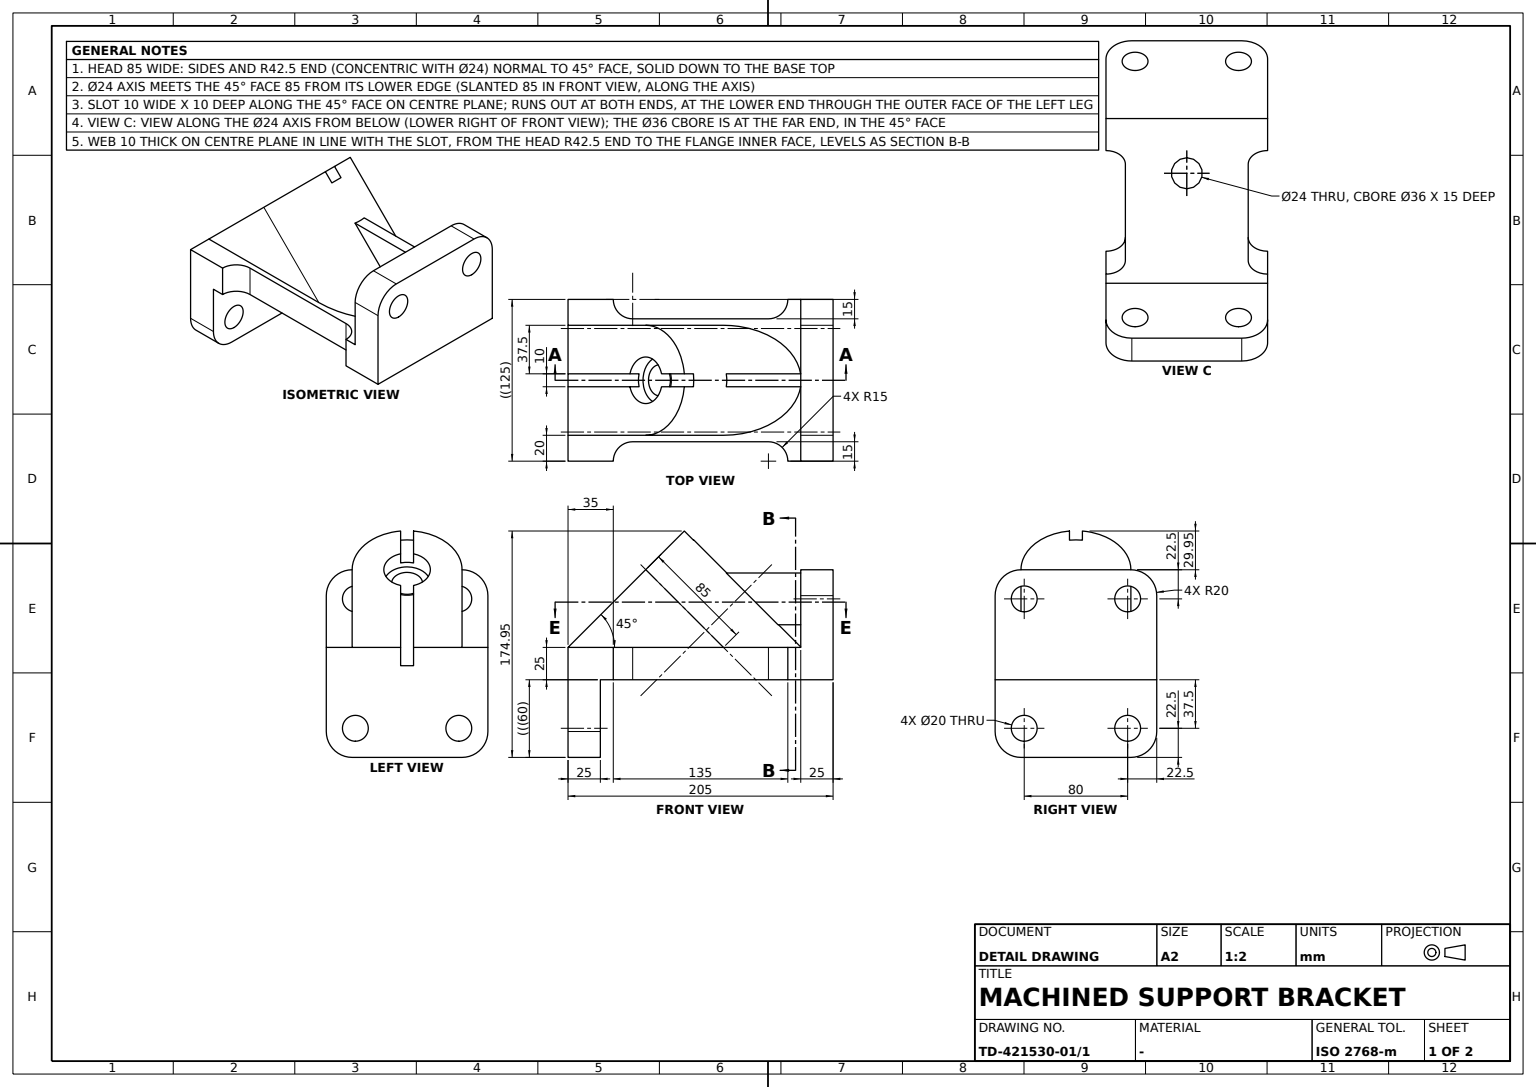
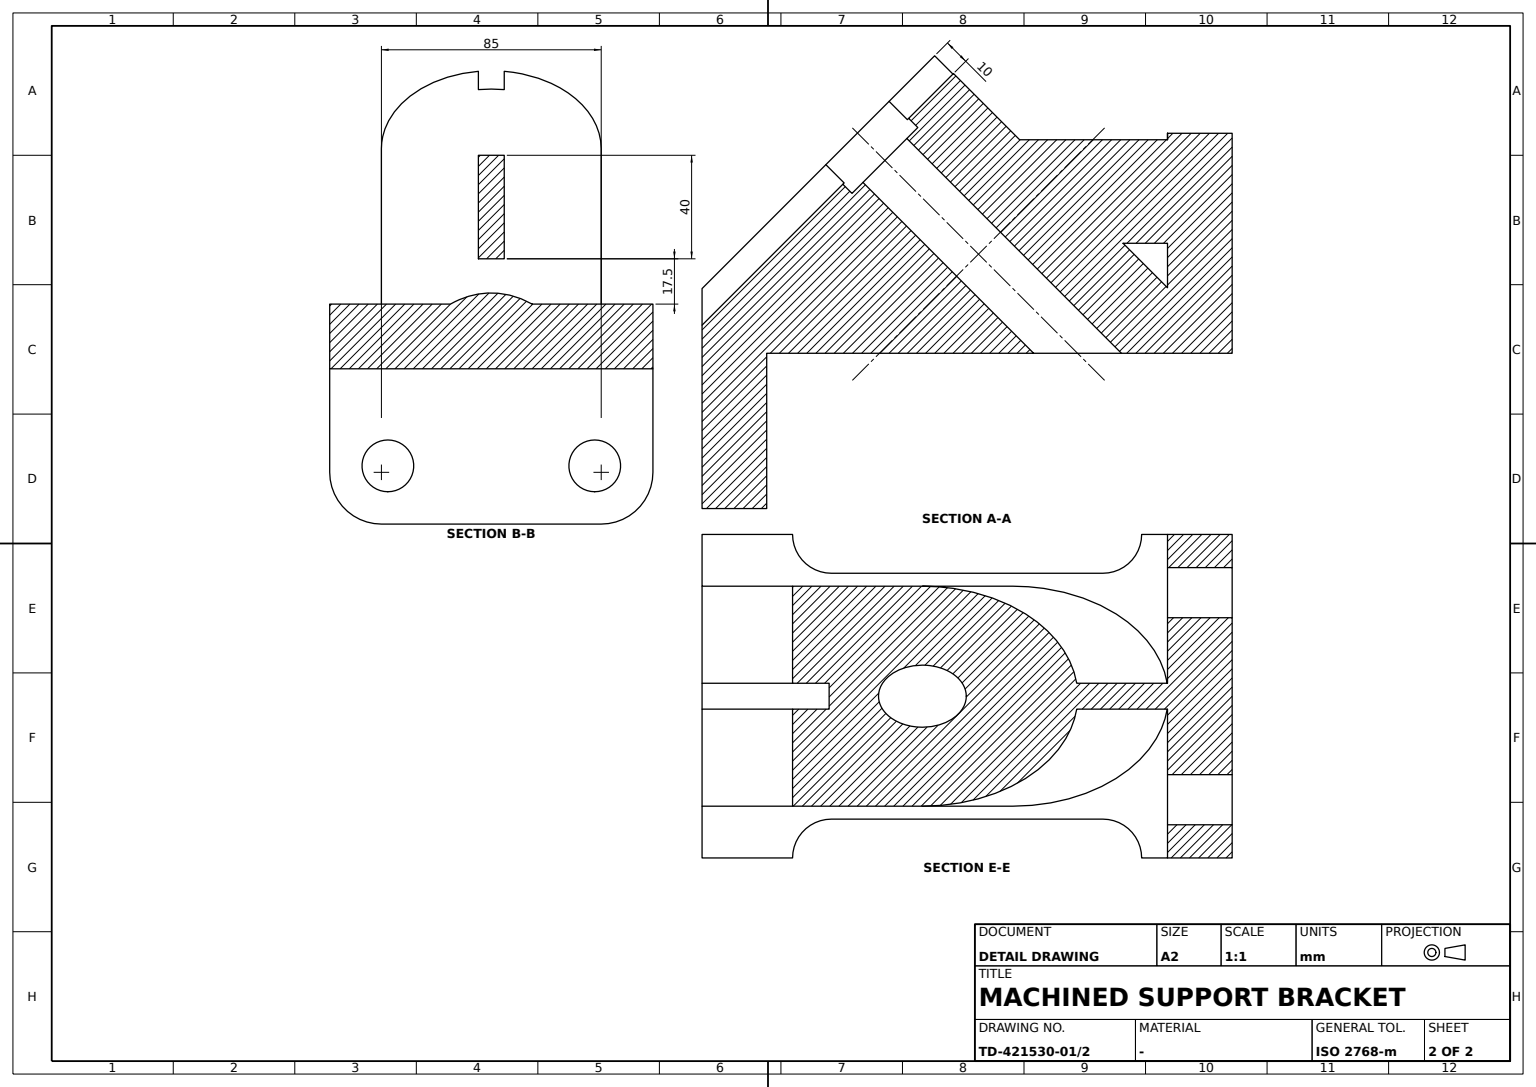
CATIA V5 part; units mm, degrees
sketch "Sketch1" plane through (0, 0, 0) normal (0, 0, 1) x (1, 0, 0)
  line L0 (-62.5, 102.5) -> (62.5, 102.5)
  line L1 (62.5, 102.5) -> (62.5, 67.5)
  line L2 (62.5, -102.5) -> (-62.5, -102.5)
  line L3 (-62.5, -102.5) -> (-62.5, -67.5)
  point P0 (62.5, -102.5)
  line L4 (62.5, 67.5) -> (62.5, 67.5)
  point P1 (62.5, 67.5)
  point P2 (47.5, 67.5)
  line L5 (47.5, 52.5) -> (47.5, -52.5)
  point P3 (47.5, -67.5)
  line L6 (62.5, -67.5) -> (62.5, -67.5)
  point P4 (62.5, -67.5)
  arc A0 (47.5, -52.5) -> (62.5, -67.5) centre (62.5, -52.5) ccw
  point P5 (47.5, -52.5)
  point P6 (62.5, -67.5)
  point P7 (62.5, -52.5)
  arc A1 (62.5, 67.5) -> (47.5, 52.5) centre (62.5, 52.5) ccw
  point P8 (62.5, 67.5)
  point P9 (47.5, 52.5)
  point P10 (62.5, -67.5)
  line L7 (62.5, -67.5) -> (62.5, -102.5)
  point P11 (62.5, 67.5)
  point P12 (-62.5, 67.5)
  point P13 (-47.5, 67.5)
  point P14 (-47.5, -67.5)
  point P15 (-62.5, -67.5)
  point P16 (-47.5, -52.5)
  point P17 (-62.5, -67.5)
  point P18 (-62.5, 67.5)
  point P19 (-47.5, 52.5)
  point P20 (-62.5, -67.5)
  point P21 (-62.5, 67.5)
  line L8 (-62.5, 67.5) -> (-62.5, 67.5)
  line L9 (-47.5, 52.5) -> (-47.5, -52.5)
  line L10 (-62.5, -67.5) -> (-62.5, -67.5)
  arc A2 (-47.5, -52.5) -> (-62.5, -67.5) centre (-62.5, -52.5) cw
  arc A3 (-62.5, 67.5) -> (-47.5, 52.5) centre (-62.5, 52.5) cw
  point P22 (-62.5, 67.5)
  line L11 (-62.5, 67.5) -> (-62.5, 102.5)
  point P23 (-62.5, -67.5)
  dimension "length L0" = 125
  dimension "distance P2 P3" = 135
  dimension "radius A0" = 15
  dimension "distance P1 P2" = 15
  dimension "radius A1" = 15
  dimension "distance P7 P0" = 50
  constraint horizontal L0 x-axis
  constraint horizontal L2 x-axis
  constraint horizontal L4 x-axis
  constraint horizontal L6 x-axis
  constraint vertical L1 y-axis
  constraint vertical L3 y-axis
  constraint vertical L5 y-axis
  constraint vertical L7 y-axis
  constraint vertical L11 y-axis
  constraint symmetry L0 L2 x-axis
  constraint symmetry L3 L1 y-axis
  constraint symmetry L4 L6 x-axis
  constraint symmetry P1 P12 y-axis
  constraint symmetry P2 P13 y-axis
  constraint symmetry P3 P14 y-axis
  constraint symmetry P4 P15 y-axis
  constraint symmetry P5 P16 y-axis
  constraint symmetry P6 P17 y-axis
  constraint symmetry P8 P18 y-axis
  constraint symmetry P9 P19 y-axis
  constraint symmetry P10 P20 y-axis
  constraint symmetry P11 P21 y-axis
  constraint symmetry L4 L8 y-axis
  constraint symmetry L5 L9 y-axis
  constraint symmetry L6 L10 y-axis
  constraint symmetry A0 A2 y-axis
  constraint symmetry A1 A3 y-axis
  constraint coincidence P1 L1
  constraint coincidence P4 L1
  constraint coincidence L5 P3
  constraint coincidence L6 P3
  constraint coincidence L4 P2
  constraint coincidence L5 P2
  constraint coincidence L6 P10
  constraint coincidence L4 P11
  constraint coincidence L1 L7
  constraint coincidence L8 P22
  constraint coincidence L10 P23
  constraint coincidence L3 L11
  constraint tangency A0 L5
  constraint tangency A0 L6
  constraint tangency A1 L4
  constraint tangency A1 L5
extrude "Pad1" add sketch "Sketch1" along normal mid plane 25
sketch "Sketch2" plane through (0, 0, 12.5) normal (0, 0, 1) x (1, 0, 0)
  point P0 (0, 90)
  line L0 (62.5, 102.5) -> (62.5, 77.5)
  line L1 (62.5, 77.5) -> (-62.5, 77.5)
  line L2 (-62.5, 77.5) -> (-62.5, 102.5)
  line L3 (-62.5, 102.5) -> (62.5, 102.5)
  line L4 (62.5, 102.5) -> (-62.5, 102.5) construction
  line L5 (62.5, 67.5) -> (62.5, 102.5) construction
  dimension "length L0" = 25
  constraint coincidence P0 y-axis
  constraint coincidence L4 L3
  constraint coincidence L0 L5
  constraint vertical L0 y-axis
  constraint vertical L2 y-axis
  constraint horizontal L1 x-axis
  constraint horizontal L3 x-axis
  constraint equidistance L0 L2 P0
  constraint equidistance L1 L3 P0
extrude "Pad2" add sketch "Sketch2" along normal blind 60
sketch "Sketch3" plane through (0, 0, -12.5) normal (0, 0, -1) x (1, 0, 0)
  point P0 (0, 90)
  line L0 (62.5, 102.5) -> (62.5, 77.5)
  line L1 (62.5, 77.5) -> (-62.5, 77.5)
  line L2 (-62.5, 77.5) -> (-62.5, 102.5)
  line L3 (-62.5, 102.5) -> (62.5, 102.5)
  line L4 (-62.5, 102.5) -> (62.5, 102.5) construction
  line L5 (62.5, 102.5) -> (62.5, 67.5) construction
  dimension "length L0" = 25
  constraint coincidence P0 y-axis
  constraint coincidence L4 L3
  constraint coincidence L0 L5
  constraint vertical L0 y-axis
  constraint vertical L2 y-axis
  constraint horizontal L1 x-axis
  constraint horizontal L3 x-axis
  constraint equidistance L0 L2 P0
  constraint equidistance L1 L3 P0
extrude "Pad3" add sketch "Sketch3" along normal blind 60
fillet "Fillet1" radius 20 4 edges at (62.5, 90, 72.5) (-62.5, 90, 72.5) (-62.5, -90, -72.5) (62.5, -90, -72.5)
sketch "Sketch4" plane through (0, 0, 0) normal (0, 1, 0) x (-1, 0, 0)
  circle A0 centre (40, 50) radius 10
  circle A1 centre (-40, 50) radius 10
  circle A2 centre (40, -50) radius 10
  circle A3 centre (-40, -50) radius 10
  dimension "radius A0" = 10
  dimension "radius A2" = 10
  constraint symmetry A0 A1 y-axis
  constraint symmetry A2 A3 y-axis
extrude "Pocket1" cut sketch "Sketch4" along normal mid plane 400
ref_plane "Plane1" through (0, -57.5, 57.5) normal (0, 0.7071, -0.7071) x (-1, 0, 0)
sketch "Sketch5" plane through (0, -57.5, 57.5) normal (0, 0.7071, -0.7071) x (-1, 0, 0)
  point P0 (0, -21.1396)
  line L0 (42.5, 21.3604) -> (42.5, -63.6396)
  line L1 (42.5, -63.6396) -> (-42.5, -63.6396)
  line L2 (-42.5, -63.6396) -> (-42.5, 21.3604)
  line L3 (62.5, -63.6396) -> (-62.5, -63.6396) construction
  arc A0 (42.5, 21.3604) -> (-42.5, 21.3604) centre (0, 21.3604) ccw
  dimension "length L0" = 85
  dimension "radius A0" = 42.5
  constraint coincidence P0 y-axis
  constraint coincidence L1 L3
  constraint vertical L0 y-axis
  constraint vertical L2 y-axis
  constraint horizontal L1 x-axis
  constraint equidistance L0 L2 P0
  constraint tangency A0 L0
extrude "Pad4" add sketch "Sketch5" along normal up to surface surface through (0, 0, 12.5) normal (0, 0, 1)
sketch "Sketch6" plane through (0, -57.5, 57.5) normal (0, -0.7071, 0.7071) x (1, 0, 0)
  line L0 (5, 80) -> (5, -80)
  line L1 (5, -80) -> (-5, -80)
  line L2 (-5, -80) -> (-5, 80)
  line L3 (-5, 80) -> (5, 80)
  dimension "distance L2 L0" = 10
  constraint vertical L0 y-axis
  constraint vertical L2 y-axis
  constraint horizontal L1 x-axis
  constraint horizontal L3 x-axis
  constraint equidistance L0 L2 origin
  constraint equidistance L1 L3 origin
  constraint symmetry L2 L0 y-axis
extrude "Pocket2" cut sketch "Sketch6" against normal blind 10
sketch "Sketch7" plane through (-29.0628, -42.8592, 72.1408) normal (0, -0.7071, 0.7071) x (1, 0, 0)
  point P0 (29.0628, 0.6551)
  arc A0 (71.5628, 0.6551) -> (-13.4372, 0.6551) centre (29.0628, 0.6551) ccw construction
  constraint concentricity A0 P0
hole "Hole1" at (0, -42.3959, 72.6041) direction (0, 0.7071, -0.7071) diameter 24 end through all counterbore diameter 36 counterbore depth 15
sketch "Sketch8" plane through (0, 77.5, 0) normal (0, -1, 0) x (1, 0, 0)
  point P0 (0, 50)
  line L0 (5, 70) -> (5, 30)
  line L1 (5, 30) -> (-5, 30)
  line L2 (-5, 30) -> (-5, 70)
  line L3 (-5, 70) -> (5, 70)
  dimension "length L0" = 40
  dimension "length L3" = 10
  constraint coincidence P0 y-axis
  constraint vertical L0 y-axis
  constraint vertical L2 y-axis
  constraint horizontal L1 x-axis
  constraint horizontal L3 x-axis
  constraint equidistance L0 L2 P0
  constraint equidistance L1 L3 P0
extrude "Pad5" add sketch "Sketch8" along normal up to surface face at (-37.4554, 45.9052, 12.7052)
